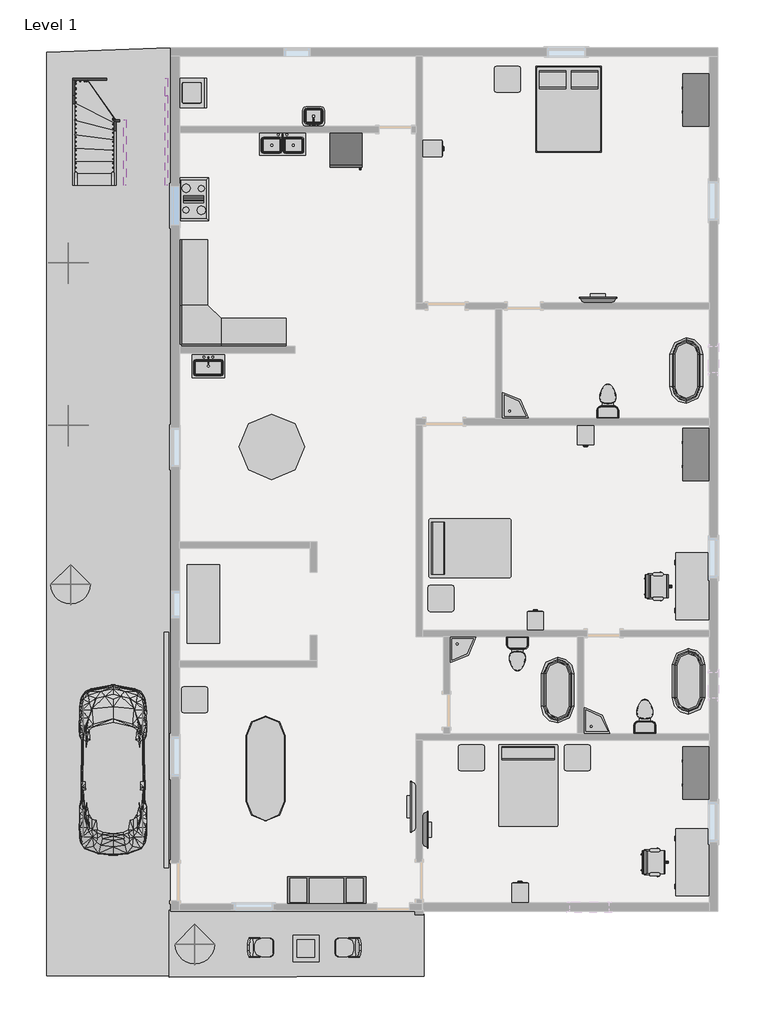
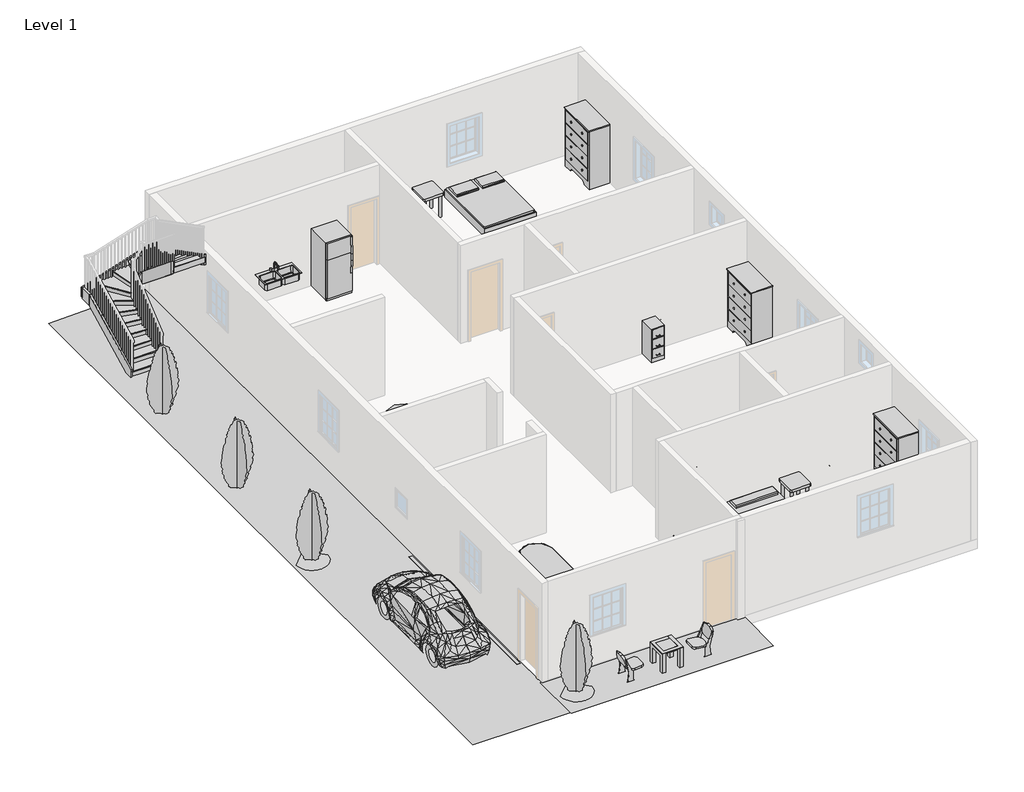
# One storey, part 3 of 3: 30 furniture elements, 16 flow terminals, 8 members, 7 proxies, 4 geographic elements, 1 stair flight.
"""IFC4 building model written with IfcOpenShell, lengths in millimetres."""

from ifc_helpers import new_model, si_unit, frame, origin, place, context, project, spatial, polyline, outline, extrude, triangles, transform, mapped, element, save
from components import proxy_bb1e6e30, parking_space_9_x_18_90_deg_b8b21359, rpc_beetle_rpc_beetle_3ce7ba48, proxy_a13a33b2, proxy_718fa39f, flow_terminal_accce45a, flow_terminal_bd5cdcf8, flow_terminal_a53be723, flow_terminal_38af2918, flow_terminal_62a433f7, toilet_domestic_3d_toilet_domestic_3d_f7549cf7, toilet_domestic_3d_toilet_domestic_3d_183bbd19, flow_terminal_b374fae2, furniture_1d2926bd, furniture_0253826f, furniture_552c1472, chair_task_arms_chair_task_arms_fa5a08ef, furniture_013ab306, furniture_9fa109b2, furniture_cf0b6580, furniture_3d1d9cbc, furniture_56245f3a, furniture_d9bcc661, furniture_b5c51a22, furniture_e05f6f82, furniture_bbcc68ce, furniture_bcf351fa, furniture_a5b052b6, furniture_45e3acac, rpc_tree_conifer_chinese_juniper_7_1b9786cd, stair_flight_3c83121e

model = new_model("IFC4")

# Units and contexts
model_context = context("Model", 3, world=origin())
ifc_project = project(units=[si_unit("LENGTHUNIT", "METRE", prefix="MILLI")], contexts=[model_context])

# Site, building, storey
site = spatial("IfcSite", under=ifc_project)
building = spatial("IfcBuilding", under=site)
storey = spatial("IfcBuildingStorey", under=building, Name="Level 1", Elevation=0.0)

# Proxies
placement = place(None, origin())
element("IfcBuildingElementProxy", 1, Name="Building Element Proxy", at=placement, inside=storey, context=model_context, shape_type="Tessellation", body=[
    triangles([(-11126.0162292, -5278.538269, 0.0), (-5181.8354507, -5380.1378815, 0.0), (-5181.8354507, -6815.2380753, 0.0), (-11126.0162292, -6841.2184662, 0.0), (-5207.2356445, -5303.9378815, 0.0), (-5448.5354507, -5278.538269, 0.0), (-11096.8610321, -5272.1880753, 0.0), (-9567.1218475, -5278.538269, 0.0)], [[4, 8, 7], [8, 4, 3], [7, 1, 4], [8, 6, 7], [3, 2, 6], [5, 6, 2], [3, 6, 8]], closed=False),
])
element("IfcBuildingElementProxy", 2, Name="Building Element Proxy", at=placement, inside=storey, context=model_context, shape_type="Tessellation", body=[
    triangles([(-11087.3360321, 14812.8621185, 0.0), (-13982.9360321, 14711.2625061, 0.0), (-11100.035257, -6815.2380753, 0.0), (-13982.9360321, -6802.538269, 0.0)], [[2, 4, 3], [3, 1, 2]], closed=False),
])
proxy_shape = proxy_bb1e6e30(model_context)
element("IfcBuildingElementProxy", 3, Name="Cook Top-4 Unit : 36\" x 20\"", ObjectType="Cook Top-4 Unit : 36\" x 20\"", at=placement, inside=storey, context=model_context, shape_type="MappedRepresentation", body=[
    mapped(proxy_shape, transform((-10553.9357228, 11282.2620171, 0.0), x_axis=(0.0, 1.0000000000000002, 0.0), y_axis=(-1.0000000000000002, 0.0, 0.0), z_axis=(0.0, 0.0, 1.0))),
])
parking_space_9_x_18_90_deg_shape = parking_space_9_x_18_90_deg_b8b21359(model_context)
element("IfcBuildingElementProxy", 4, Name="Parking Space : 9' x 18' - 90 deg", ObjectType="Parking Space : 9' x 18' - 90 deg", at=placement, inside=storey, context=model_context, shape_type="MappedRepresentation", body=[
    mapped(parking_space_9_x_18_90_deg_shape, transform((-11188.9357228, -4287.9379829, 0.0), x_axis=(-1.0, 0.0, 0.0), y_axis=(0.0, -1.0, 0.0), z_axis=(0.0, 0.0, 1.0))),
])
rpc_beetle_rpc_beetle_shape = rpc_beetle_rpc_beetle_3ce7ba48(model_context)
element("IfcBuildingElementProxy", 5, Name="RPC Beetle : RPC Beetle", ObjectType="RPC Beetle : RPC Beetle", at=placement, inside=storey, context=model_context, shape_type="MappedRepresentation", body=[
    mapped(rpc_beetle_rpc_beetle_shape, transform((-12433.5357228, -3246.5379829, 0.0), x_axis=(1.0000000000000007, 0.0, 0.0), y_axis=(0.0, 1.0000000000000007, 0.0), z_axis=(0.0, 0.0, 1.0))),
])
proxy_2_shape = proxy_a13a33b2(model_context)
element("IfcBuildingElementProxy", 6, Name="Refrigerator : 30\" x 32\" RH", ObjectType="Refrigerator : 30\" x 32\" RH", at=placement, inside=storey, context=model_context, shape_type="MappedRepresentation", body=[
    mapped(proxy_2_shape, transform((-7005.8732228, 12443.1130456, 0.0), x_axis=(1.0000000000000009, 0.0, 0.0), y_axis=(0.0, 1.0000000000000009, 0.0), z_axis=(0.0, 0.0, 1.0))),
])
proxy_3_shape = proxy_718fa39f(model_context)
element("IfcBuildingElementProxy", 7, Name="Washer : 27\" x 25\" x 35\"", ObjectType="Washer : 27\" x 25\" x 35\"", at=placement, inside=storey, context=model_context, shape_type="MappedRepresentation", body=[
    mapped(proxy_3_shape, transform((-10845.7852876, 14179.1794856, 0.0), x_axis=(0.0, -1.0000000000000004, 0.0), y_axis=(1.0000000000000004, 0.0, 0.0), z_axis=(0.0, 0.0, 1.0))),
])

# Flow terminals
flow_terminal_shape = flow_terminal_accce45a(model_context)
element("IfcFlowTerminal", 8, ObjectType="Floor Drain - Round : 5\" Strainer - 2\" Drain", at=placement, inside=storey, context=model_context, shape_type="MappedRepresentation", body=[
    mapped(flow_terminal_shape, transform((-10630.1357228, 14330.2620171, 0.0), x_axis=(1.0, 0.0, 0.0), y_axis=(0.0, 1.0, 0.0), z_axis=(0.0, 0.0, 1.0))),
])
element("IfcFlowTerminal", 9, ObjectType="Floor Drain - Round : 5\" Strainer - 2\" Drain", at=placement, inside=storey, context=model_context, shape_type="MappedRepresentation", body=[
    mapped(flow_terminal_shape, transform((230.9261263, 6530.9872371, 0.0), x_axis=(1.0, 0.0, 0.0), y_axis=(0.0, 1.0, 0.0), z_axis=(0.0, 0.0, 1.0))),
])
element("IfcFlowTerminal", 10, ObjectType="Floor Drain - Round : 5\" Strainer - 2\" Drain", at=placement, inside=storey, context=model_context, shape_type="MappedRepresentation", body=[
    mapped(flow_terminal_shape, transform((596.6642772, -833.5379829, 0.0), x_axis=(1.0, 0.0, 0.0), y_axis=(0.0, 1.0, 0.0), z_axis=(0.0, 0.0, 1.0))),
])
element("IfcFlowTerminal", 11, ObjectType="Floor Drain - Round : 5\" Strainer - 2\" Drain", at=placement, inside=storey, context=model_context, shape_type="MappedRepresentation", body=[
    mapped(flow_terminal_shape, transform((-2705.3357228, -909.7379829, 0.0), x_axis=(1.0, 0.0, 0.0), y_axis=(0.0, 1.0, 0.0), z_axis=(0.0, 0.0, 1.0))),
])
flow_terminal_2_shape = flow_terminal_bd5cdcf8(model_context)
element("IfcFlowTerminal", 12, ObjectType="Sink - Corner Floor : 24\"", at=placement, inside=storey, context=model_context, shape_type="MappedRepresentation", body=[
    mapped(flow_terminal_2_shape, transform((-3365.7357228, 6176.8620171, 609.6), x_axis=(1.0, 0.0, 0.0), y_axis=(0.0, 1.0, 0.0), z_axis=(0.0, 0.0, 1.0))),
])
element("IfcFlowTerminal", 13, ObjectType="Sink - Corner Floor : 24\"", at=placement, inside=storey, context=model_context, shape_type="MappedRepresentation", body=[
    mapped(flow_terminal_2_shape, transform((-4584.9357228, 1096.8620171, 609.6), x_axis=(0.0, -1.0000000000000004, 0.0), y_axis=(1.0000000000000004, 0.0, 0.0), z_axis=(0.0, 0.0, 1.0))),
])
element("IfcFlowTerminal", 14, ObjectType="Sink - Corner Floor : 24\"", at=placement, inside=storey, context=model_context, shape_type="MappedRepresentation", body=[
    mapped(flow_terminal_2_shape, transform((-1460.7357228, -1163.7379829, 609.6), x_axis=(1.0000000000000002, 0.0, 0.0), y_axis=(0.0, 1.0000000000000002, 0.0), z_axis=(0.0, 0.0, 1.0))),
])
flow_terminal_3_shape = flow_terminal_a53be723(model_context)
element("IfcFlowTerminal", 15, ObjectType="Sink Kitchen-Double : 42\" x 21\"", at=placement, inside=storey, context=model_context, shape_type="MappedRepresentation", body=[
    mapped(flow_terminal_3_shape, transform((-8499.5249633, 12575.316616, 0.0), x_axis=(1.0, 0.0, 0.0), y_axis=(0.0, 1.0, 0.0), z_axis=(0.0, 0.0, 1.0))),
])
flow_terminal_4_shape = flow_terminal_38af2918(model_context)
element("IfcFlowTerminal", 16, ObjectType="Sink Kitchen-Single : 30\" x 21\"", at=placement, inside=storey, context=model_context, shape_type="MappedRepresentation", body=[
    mapped(flow_terminal_4_shape, transform((-10226.7249633, 7393.716616, 0.0), x_axis=(1.0, 0.0, 0.0), y_axis=(0.0, 1.0, 0.0), z_axis=(0.0, 0.0, 1.0))),
])
flow_terminal_5_shape = flow_terminal_62a433f7(model_context)
element("IfcFlowTerminal", 17, ObjectType="Sink Vanity-Square : 20\" x 18\"", at=placement, inside=storey, context=model_context, shape_type="MappedRepresentation", body=[
    mapped(flow_terminal_5_shape, transform((-7744.2464822, 13164.2074182, 0.0), x_axis=(-1.0000000000000004, 0.0, 0.0), y_axis=(0.0, -1.0000000000000004, 0.0), z_axis=(0.0, 0.0, 1.0))),
])
toilet_domestic_3d_toilet_domestic_3d_shape = toilet_domestic_3d_toilet_domestic_3d_f7549cf7(model_context)
toilet_domestic_3d_toilet_domestic_3d_2_shape = toilet_domestic_3d_toilet_domestic_3d_183bbd19(model_context)
element("IfcFlowTerminal", 18, ObjectType="Toilet-Domestic-3D : Toilet-Domestic-3D", at=placement, inside=storey, context=model_context, shape_type="MappedRepresentation", body=[
    mapped(toilet_domestic_3d_toilet_domestic_3d_shape, transform((-901.9357228, 6671.5580445, 0.0), x_axis=(-0.9999999999999998, 0.0, 0.0), y_axis=(0.0, -0.9999999999999998, 0.0), z_axis=(0.0, 0.0, 1.0))),
    mapped(toilet_domestic_3d_toilet_domestic_3d_2_shape, transform((-901.9357228, 6671.5580445, 0.0), x_axis=(-0.9999999999999998, 0.0, 0.0), y_axis=(0.0, -0.9999999999999998, 0.0), z_axis=(0.0, 0.0, 1.0))),
])
element("IfcFlowTerminal", 19, ObjectType="Toilet-Domestic-3D : Toilet-Domestic-3D", at=placement, inside=storey, context=model_context, shape_type="MappedRepresentation", body=[
    mapped(toilet_domestic_3d_toilet_domestic_3d_shape, transform((-3010.1357228, 602.1659898, 0.0), x_axis=(1.0, 0.0, 0.0), y_axis=(0.0, 1.0, 0.0), z_axis=(0.0, 0.0, 1.0))),
    mapped(toilet_domestic_3d_toilet_domestic_3d_2_shape, transform((-3010.1357228, 602.1659898, 0.0), x_axis=(1.0, 0.0, 0.0), y_axis=(0.0, 1.0, 0.0), z_axis=(0.0, 0.0, 1.0))),
])
element("IfcFlowTerminal", 20, ObjectType="Toilet-Domestic-3D : Toilet-Domestic-3D", at=placement, inside=storey, context=model_context, shape_type="MappedRepresentation", body=[
    mapped(toilet_domestic_3d_toilet_domestic_3d_shape, transform((-38.3357228, -669.0419555, 0.0), x_axis=(-1.0000000000000004, 0.0, 0.0), y_axis=(0.0, -1.0000000000000004, 0.0), z_axis=(0.0, 0.0, 1.0))),
    mapped(toilet_domestic_3d_toilet_domestic_3d_2_shape, transform((-38.3357228, -669.0419555, 0.0), x_axis=(-1.0000000000000004, 0.0, 0.0), y_axis=(0.0, -1.0000000000000004, 0.0), z_axis=(0.0, 0.0, 1.0))),
])
flow_terminal_6_shape = flow_terminal_b374fae2(model_context)
element("IfcFlowTerminal", 21, ObjectType="Tub-Free Standing-3D : 30\" x 60\"", at=placement, inside=storey, context=model_context, shape_type="MappedRepresentation", body=[
    mapped(flow_terminal_6_shape, transform((926.8642772, 7294.4620171, 0.0), x_axis=(1.0, 0.0, 0.0), y_axis=(0.0, 1.0, 0.0), z_axis=(0.0, 0.0, 1.0))),
])
element("IfcFlowTerminal", 22, ObjectType="Tub-Free Standing-3D : 30\" x 60\"", at=placement, inside=storey, context=model_context, shape_type="MappedRepresentation", body=[
    mapped(flow_terminal_6_shape, transform((-2070.3357228, -147.7379829, 0.0), x_axis=(1.0, 0.0, 0.0), y_axis=(0.0, 1.0, 0.0), z_axis=(0.0, 0.0, 1.0))),
])
element("IfcFlowTerminal", 23, ObjectType="Tub-Free Standing-3D : 30\" x 60\"", at=placement, inside=storey, context=model_context, shape_type="MappedRepresentation", body=[
    mapped(flow_terminal_6_shape, transform((977.6642772, 55.4620171, 0.0), x_axis=(1.0, 0.0, 0.0), y_axis=(0.0, 1.0, 0.0), z_axis=(0.0, 0.0, 1.0))),
])

# Furniture
furniture_shape = furniture_1d2926bd(model_context)
element("IfcFurniture", 24, ObjectType="Bed-Box : Queen 60\" x 79\"", at=placement, inside=storey, context=model_context, shape_type="MappedRepresentation", body=[
    mapped(furniture_shape, transform((-2155.4881818, 13612.1915253, 0.0), x_axis=(1.0, 0.0, 0.0), y_axis=(0.0, 1.0, 0.0), z_axis=(0.0, 0.0, 1.0))),
])
furniture_2_shape = furniture_0253826f(model_context)
element("IfcFurniture", 25, ObjectType="Bed-Standard.0001 : Double 54\" x 75\"", at=placement, inside=storey, context=model_context, shape_type="MappedRepresentation", body=[
    mapped(furniture_2_shape, transform((-4160.6308048, 2882.7734925, 0.0), x_axis=(0.0, 1.0000000000000002, 0.0), y_axis=(-1.0000000000000002, 0.0, 0.0), z_axis=(0.0, 0.0, 1.0))),
])
element("IfcFurniture", 26, ObjectType="Bed-Standard.0001 : Double 54\" x 75\"", at=placement, inside=storey, context=model_context, shape_type="MappedRepresentation", body=[
    mapped(furniture_2_shape, transform((-3027.6242474, -2324.6429009, 0.0), x_axis=(1.0, 0.0, 0.0), y_axis=(0.0, 1.0, 0.0), z_axis=(0.0, 0.0, 1.0))),
])
furniture_3_shape = furniture_552c1472(model_context)
element("IfcFurniture", 27, ObjectType="Cabinet-File 3 Drawer : 15\" x 18\"", at=placement, inside=storey, context=model_context, shape_type="MappedRepresentation", body=[
    mapped(furniture_3_shape, transform((-5133.4700229, 12591.2584641, 0.0), x_axis=(0.0, 1.0000000000000002, 0.0), y_axis=(-1.0000000000000002, 0.0, 0.0), z_axis=(0.0, 0.0, 1.0))),
])
element("IfcFurniture", 28, ObjectType="Cabinet-File 3 Drawer : 15\" x 18\"", at=placement, inside=storey, context=model_context, shape_type="MappedRepresentation", body=[
    mapped(furniture_3_shape, transform((-2718.9321698, 1310.327717, 0.0), x_axis=(-1.0000000000000002, 0.0, 0.0), y_axis=(0.0, -1.0000000000000002, 0.0), z_axis=(0.0, 0.0, 1.0))),
])
element("IfcFurniture", 29, ObjectType="Cabinet-File 3 Drawer : 15\" x 18\"", at=placement, inside=storey, context=model_context, shape_type="MappedRepresentation", body=[
    mapped(furniture_3_shape, transform((-1294.7392757, 5937.9963172, 0.0), x_axis=(1.0, 0.0, 0.0), y_axis=(0.0, 1.0, 0.0), z_axis=(0.0, 0.0, 1.0))),
])
element("IfcFurniture", 30, ObjectType="Cabinet-File 3 Drawer : 15\" x 18\"", at=placement, inside=storey, context=model_context, shape_type="MappedRepresentation", body=[
    mapped(furniture_3_shape, transform((-3074.5321698, -5014.272283, 0.0), x_axis=(-1.0, 0.0, 0.0), y_axis=(0.0, -1.0, 0.0), z_axis=(0.0, 0.0, 1.0))),
])
chair_task_arms_chair_task_arms_shape = chair_task_arms_chair_task_arms_fa5a08ef(model_context)
element("IfcFurniture", 31, ObjectType="Chair-Task Arms : Chair-Task Arms", at=placement, inside=storey, context=model_context, shape_type="MappedRepresentation", body=[
    mapped(chair_task_arms_chair_task_arms_shape, transform((222.1183756, 2406.2528368, 0.0), x_axis=(0.0, -1.0000000000000004, 0.0), y_axis=(1.0000000000000004, 0.0, 0.0), z_axis=(0.0, 0.0, 1.0))),
])
element("IfcFurniture", 32, ObjectType="Chair-Task Arms : Chair-Task Arms", at=placement, inside=storey, context=model_context, shape_type="MappedRepresentation", body=[
    mapped(chair_task_arms_chair_task_arms_shape, transform((145.9183756, -4019.9471632, 0.0), x_axis=(0.0, -1.0000000000000004, 0.0), y_axis=(1.0000000000000004, 0.0, 0.0), z_axis=(0.0, 0.0, 1.0))),
])
furniture_4_shape = furniture_013ab306(model_context)
element("IfcFurniture", 33, ObjectType="Desk : 60\" x 30\"", at=placement, inside=storey, context=model_context, shape_type="MappedRepresentation", body=[
    mapped(furniture_4_shape, transform((698.2642772, 3027.2620171, 0.0), x_axis=(0.0, -1.0000000000000007, 0.0), y_axis=(1.0000000000000007, 0.0, 0.0), z_axis=(0.0, 0.0, 1.0))),
])
element("IfcFurniture", 34, ObjectType="Desk : 60\" x 30\"", at=placement, inside=storey, context=model_context, shape_type="MappedRepresentation", body=[
    mapped(furniture_4_shape, transform((698.2642772, -3398.9379829, 0.0), x_axis=(0.0, -1.0000000000000004, 0.0), y_axis=(1.0000000000000004, 0.0, 0.0), z_axis=(0.0, 0.0, 1.0))),
])
furniture_5_shape = furniture_9fa109b2(model_context)
element("IfcFurniture", 35, ObjectType="Dresser : 48\" x 72\" x 24\"", at=placement, inside=storey, context=model_context, shape_type="MappedRepresentation", body=[
    mapped(furniture_5_shape, transform((1518.6272313, 13324.4687573, 0.0), x_axis=(0.0, -1.0000000000000007, 0.0), y_axis=(1.0000000000000007, 0.0, 0.0), z_axis=(0.0, 0.0, 1.0))),
])
element("IfcFurniture", 36, ObjectType="Dresser : 48\" x 72\" x 24\"", at=placement, inside=storey, context=model_context, shape_type="MappedRepresentation", body=[
    mapped(furniture_5_shape, transform((1518.6272313, 5069.4687573, 0.0), x_axis=(0.0, -1.0000000000000007, 0.0), y_axis=(1.0000000000000007, 0.0, 0.0), z_axis=(0.0, 0.0, 1.0))),
])
element("IfcFurniture", 37, ObjectType="Dresser : 48\" x 72\" x 24\"", at=placement, inside=storey, context=model_context, shape_type="MappedRepresentation", body=[
    mapped(furniture_5_shape, transform((1518.6272313, -2347.3312427, 0.0), x_axis=(0.0, -1.0000000000000007, 0.0), y_axis=(1.0000000000000007, 0.0, 0.0), z_axis=(0.0, 0.0, 1.0))),
])
furniture_6_shape = furniture_cf0b6580(model_context)
element("IfcFurniture", 38, ObjectType="Entertainment Center : 72\" x 72\" x 24\"", at=placement, inside=storey, context=model_context, shape_type="MappedRepresentation", body=[
    mapped(furniture_6_shape, transform((-7455.1357228, -4389.5379829, 0.0), x_axis=(1.0, 0.0, 0.0), y_axis=(0.0, 1.0, 0.0), z_axis=(0.0, 0.0, 1.0))),
])
furniture_7_shape = furniture_3d1d9cbc(model_context)
element("IfcFurniture", 39, ObjectType="Seating-Auditorium : 18\" x 24\" x 30\"", at=placement, inside=storey, context=model_context, shape_type="MappedRepresentation", body=[
    mapped(furniture_7_shape, transform((-9194.4111326, -5981.410114, 0.0), x_axis=(0.0, -1.0000000000000007, 0.0), y_axis=(1.0000000000000007, 0.0, 0.0), z_axis=(0.0, 0.0, 1.0))),
])
element("IfcFurniture", 40, ObjectType="Seating-Auditorium : 18\" x 24\" x 30\"", at=placement, inside=storey, context=model_context, shape_type="MappedRepresentation", body=[
    mapped(furniture_7_shape, transform((-6757.2603129, -6302.8658517, 0.0), x_axis=(0.0, 1.000000000000001, 0.0), y_axis=(-1.000000000000001, 0.0, 0.0), z_axis=(0.0, 0.0, 1.0))),
])
furniture_8_shape = furniture_56245f3a(model_context)
element("IfcFurniture", 41, ObjectType="TV - Flat Screen : 32\"", at=placement, inside=storey, context=model_context, shape_type="MappedRepresentation", body=[
    mapped(furniture_8_shape, transform((-5161.3970991, -3394.9934687, 914.4), x_axis=(0.0, 1.0, 0.0), y_axis=(-1.0, 0.0, 0.0), z_axis=(0.0, 0.0, 1.0))),
])
element("IfcFurniture", 42, ObjectType="TV - Flat Screen : 32\"", at=placement, inside=storey, context=model_context, shape_type="MappedRepresentation", body=[
    mapped(furniture_8_shape, transform((-1134.4802369, 8927.8006408, 914.4), x_axis=(-1.0, 0.0, 0.0), y_axis=(0.0, -1.0, 0.0), z_axis=(0.0, 0.0, 1.0))),
])
furniture_9_shape = furniture_d9bcc661(model_context)
element("IfcFurniture", 43, ObjectType="TV - Flat Screen : 46\"", at=placement, inside=storey, context=model_context, shape_type="MappedRepresentation", body=[
    mapped(furniture_9_shape, transform((-5430.8743464, -2869.482497, 0.0), x_axis=(0.0, -1.0000000000000004, 0.0), y_axis=(1.0000000000000004, 0.0, 0.0), z_axis=(0.0, 0.0, 1.0))),
])
furniture_10_shape = furniture_b5c51a22(model_context)
element("IfcFurniture", 44, ObjectType="Table-Coffee : 24\" x 24\" x 24\"", at=placement, inside=storey, context=model_context, shape_type="MappedRepresentation", body=[
    mapped(furniture_10_shape, transform((-7956.0014895, -6262.7490607, 0.0), x_axis=(1.0, 0.0, 0.0), y_axis=(0.0, 1.0, 0.0), z_axis=(0.0, 0.0, 1.0))),
])
furniture_11_shape = furniture_e05f6f82(model_context)
element("IfcFurniture", 45, ObjectType="Table-Dining Oval : 36\" x 96\" Glass Top", at=placement, inside=storey, context=model_context, shape_type="MappedRepresentation", body=[
    mapped(furniture_11_shape, transform((-9235.6340834, -1574.7183108, 0.0), x_axis=(0.0, 1.0000000000000002, 0.0), y_axis=(-1.0000000000000002, 0.0, 0.0), z_axis=(0.0, 0.0, 1.0))),
])
furniture_12_shape = furniture_bbcc68ce(model_context)
element("IfcFurniture", 46, ObjectType="Table-Dining Round w Chairs : 60\" Diameter", at=placement, inside=storey, context=model_context, shape_type="MappedRepresentation", body=[
    mapped(furniture_12_shape, transform((-8837.1230967, 5701.3407056, 0.0), x_axis=(1.0, 0.0, 0.0), y_axis=(0.0, 1.0, 0.0), z_axis=(0.0, 0.0, 1.0))),
])
furniture_13_shape = furniture_bcf351fa(model_context)
element("IfcFurniture", 47, ObjectType="Table-End : 24\" x 24\"", at=placement, inside=storey, context=model_context, shape_type="MappedRepresentation", body=[
    mapped(furniture_13_shape, transform((-3547.2693531, 13923.8620171, 0.0), x_axis=(1.0, 0.0, 0.0), y_axis=(0.0, 1.0, 0.0), z_axis=(0.0, 0.0, 1.0))),
])
element("IfcFurniture", 48, ObjectType="Table-End : 24\" x 24\"", at=placement, inside=storey, context=model_context, shape_type="MappedRepresentation", body=[
    mapped(furniture_13_shape, transform((-5096.6693531, 1833.4620171, 0.0), x_axis=(1.0, 0.0, 0.0), y_axis=(0.0, 1.0, 0.0), z_axis=(0.0, 0.0, 1.0))),
])
element("IfcFurniture", 49, ObjectType="Table-End : 24\" x 24\"", at=placement, inside=storey, context=model_context, shape_type="MappedRepresentation", body=[
    mapped(furniture_13_shape, transform((-4385.4693531, -1874.9379829, 0.0), x_axis=(1.0, 0.0, 0.0), y_axis=(0.0, 1.0, 0.0), z_axis=(0.0, 0.0, 1.0))),
])
element("IfcFurniture", 50, ObjectType="Table-End : 24\" x 24\"", at=placement, inside=storey, context=model_context, shape_type="MappedRepresentation", body=[
    mapped(furniture_13_shape, transform((-1921.6693531, -1874.9379829, 0.0), x_axis=(1.0, 0.0, 0.0), y_axis=(0.0, 1.0, 0.0), z_axis=(0.0, 0.0, 1.0))),
])
element("IfcFurniture", 51, ObjectType="Table-End : 24\" x 24\"", at=placement, inside=storey, context=model_context, shape_type="MappedRepresentation", body=[
    mapped(furniture_13_shape, transform((-10837.0693531, -528.7379829, 0.0), x_axis=(1.0, 0.0, 0.0), y_axis=(0.0, 1.0, 0.0), z_axis=(0.0, 0.0, 1.0))),
])
furniture_14_shape = furniture_a5b052b6(model_context)
element("IfcFurniture", 52, ObjectType="Table-Rectangular : 72\" x 30\"", at=placement, inside=storey, context=model_context, shape_type="MappedRepresentation", body=[
    mapped(furniture_14_shape, transform((-10325.3357228, 1858.8620171, 0.0), x_axis=(0.0, 1.0000000000000002, 0.0), y_axis=(-1.0000000000000002, 0.0, 0.0), z_axis=(0.0, 0.0, 1.0))),
])
furniture_15_shape = furniture_45e3acac(model_context)
element("IfcFurniture", 53, ObjectType="Work Station Cubicle : 96\" x 96\"", at=placement, inside=storey, context=model_context, shape_type="MappedRepresentation", body=[
    mapped(furniture_15_shape, transform((-11379.1587304, 7984.9937693, 0.0), x_axis=(0.0, 1.0000000000000002, 0.0), y_axis=(-1.0000000000000002, 0.0, 0.0), z_axis=(0.0, 0.0, 1.0))),
])

# Geographic elements
rpc_tree_conifer_chinese_juniper_7_shape = rpc_tree_conifer_chinese_juniper_7_1b9786cd(model_context)
element("IfcGeographicElement", 54, ObjectType="RPC Tree - Conifer : Chinese Juniper - 7'", at=placement, inside=storey, context=model_context, shape_type="MappedRepresentation", body=[
    mapped(rpc_tree_conifer_chinese_juniper_7_shape, transform((-10528.7323939, -6065.9379829, 0.0), x_axis=(1.0, 0.0, 0.0), y_axis=(0.0, 1.0, 0.0), z_axis=(0.0, 0.0, 1.0))),
])
element("IfcGeographicElement", 55, ObjectType="RPC Tree - Conifer : Chinese Juniper - 7'", at=placement, inside=storey, context=model_context, shape_type="MappedRepresentation", body=[
    mapped(rpc_tree_conifer_chinese_juniper_7_shape, transform((-13475.1323939, 9809.0620171, 0.0), x_axis=(1.0, 0.0, 0.0), y_axis=(0.0, 1.0, 0.0), z_axis=(0.0, 0.0, 1.0))),
])
element("IfcGeographicElement", 56, ObjectType="RPC Tree - Conifer : Chinese Juniper - 7'", at=placement, inside=storey, context=model_context, shape_type="MappedRepresentation", body=[
    mapped(rpc_tree_conifer_chinese_juniper_7_shape, transform((-13475.1323939, 6024.4620171, 0.0), x_axis=(1.0, 0.0, 0.0), y_axis=(0.0, 1.0, 0.0), z_axis=(0.0, 0.0, 1.0))),
])
element("IfcGeographicElement", 57, ObjectType="RPC Tree - Conifer : Chinese Juniper - 7'", at=placement, inside=storey, context=model_context, shape_type="MappedRepresentation", body=[
    mapped(rpc_tree_conifer_chinese_juniper_7_shape, transform((-13424.3323939, 2316.0620171, 0.0), x_axis=(1.0, 0.0, 0.0), y_axis=(0.0, 1.0, 0.0), z_axis=(0.0, 0.0, 1.0))),
])

# Members
element("IfcMember", 58, ObjectType="Stringer - 2\" Width", at=placement, inside=storey, context=model_context, shape_type="SweptSolid", body=[
    extrude(outline(polyline([(11608.7303252, 0.0), (11608.7303252, 229.639954), (13696.1475169, 1305.3956453), (13696.1475169, 962.500629), (11828.4926428, 0.0), (11608.7303252, 0.0)])), frame((-13373.3357228, 0.0, 0.0), z_axis=(1.0, 0.0, 0.0), x_axis=(0.0, 1.0, 0.0)), (0.0, 0.0, 1.0), 50.8),
])
element("IfcMember", 59, ObjectType="Stringer - 2\" Width", at=placement, inside=storey, context=model_context, shape_type="SweptSolid", body=[
    extrude(outline(polyline([(-13322.5357228, 13696.1475169), (-13373.3357228, 13696.1475169), (-13373.3357228, 14050.8620171), (-13322.5357228, 14050.8620171), (-13322.5357228, 13696.1475169)])), frame((0.0, 0.0, 962.500629), z_axis=(0.0, 0.0, 1.0), x_axis=(1.0, 0.0, 0.0)), (0.0, 0.0, 1.0), 342.8950162),
])
element("IfcMember", 60, ObjectType="Stringer - 2\" Width", at=placement, inside=storey, context=model_context, shape_type="SweptSolid", body=[
    extrude(outline(polyline([(1289.0952212, -13373.3357228), (1000.5956453, -13373.3357228), (1000.5956453, -13203.8132398), (1638.9682298, -11214.3357228), (1969.9972697, -11214.3357228), (1969.9972697, -11251.3158401), (1289.0952212, -13373.3357228)])), frame((0.0, 14050.8620171, 0.0), z_axis=(0.0, 1.0, 0.0), x_axis=(0.0, 0.0, 1.0)), (0.0, 0.0, 1.0), 50.8),
])
element("IfcMember", 61, ObjectType="Stringer - 2\" Width", at=placement, inside=storey, context=model_context, shape_type="SweptSolid", body=[
    extrude(outline(polyline([(-11214.3357228, 14101.6620171), (-11163.5357228, 14101.6620171), (-11163.5357228, 13696.1475169), (-11214.3357228, 13696.1475169), (-11214.3357228, 14101.6620171)])), frame((0.0, 0.0, 1649.8904473), z_axis=(0.0, 0.0, 1.0), x_axis=(1.0, 0.0, 0.0)), (0.0, 0.0, 1.0), 320.1068224),
])
element("IfcMember", 62, ObjectType="Stringer - 2\" Width", at=placement, inside=storey, context=model_context, shape_type="SweptSolid", body=[
    extrude(outline(polyline([(13696.1475169, 1969.9972697), (13696.1475169, 1649.8904473), (11608.7303252, 2725.6461385), (11608.7303252, 3045.7529609), (13696.1475169, 1969.9972697)])), frame((-11214.3357228, 0.0, 0.0), z_axis=(1.0, 0.0, 0.0), x_axis=(0.0, 1.0, 0.0)), (0.0, 0.0, 1.0), 50.8),
])
element("IfcMember", 63, ObjectType="Stringer - 2\" Width", at=placement, inside=storey, context=model_context, shape_type="SweptSolid", body=[
    extrude(outline(polyline([(11608.7303252, 0.0), (11608.7303252, 176.1764461), (13085.6620171, 1380.418648), (13085.6620171, 987.1410923), (11874.9919698, 0.0), (11608.7303252, 0.0)])), frame((-12408.1357228, 0.0, 0.0), z_axis=(1.0, 0.0, 0.0), x_axis=(0.0, 1.0, 0.0)), (0.0, 0.0, 1.0), 50.8),
])
element("IfcMember", 64, ObjectType="Stringer - 2\" Width", at=placement, inside=storey, context=model_context, shape_type="SweptSolid", body=[
    extrude(outline(polyline([(1573.2682978, -12408.1357228), (1028.5617647, -12408.1357228), (1028.5617647, -12373.8935055), (1360.465107, -12179.5357228), (1926.1409689, -12179.5357228), (1926.1409689, -12201.4986054), (1573.2682978, -12408.1357228)])), frame((0.0, 13085.6620171, 0.0), z_axis=(0.0, 1.0, 0.0), x_axis=(0.0, 0.0, 1.0)), (0.0, 0.0, 1.0), 50.8),
])
element("IfcMember", 65, ObjectType="Stringer - 2\" Width", at=placement, inside=storey, context=model_context, shape_type="SweptSolid", body=[
    extrude(outline(polyline([(13136.4620171, 1926.1409689), (13136.4620171, 1532.8634131), (11608.7303252, 2778.5262875), (11608.7303252, 3171.8038432), (13136.4620171, 1926.1409689)])), frame((-12179.5357228, 0.0, 0.0), z_axis=(1.0, 0.0, 0.0), x_axis=(0.0, 1.0, 0.0)), (0.0, 0.0, 1.0), 50.8),
])

# Stair flight
stair_flight_shape = stair_flight_3c83121e(model_context)
element("IfcStairFlight", 66, ObjectType="2\" Tread 1\" Nosing 1/4\" Riser", at=placement, inside=storey, context=model_context, shape_type="MappedRepresentation", body=[
    mapped(stair_flight_shape, transform((0.0, 0.0, 0.0), x_axis=(1.0, 0.0, 0.0), y_axis=(0.0, 1.0, 0.0), z_axis=(0.0, 0.0, 1.0))),
])

save(model, "model.ifc")

# Revit data of these elements
# Type "Cook Top-4 Unit : 36\" x 20\""
#   Assembly Code = "E1090400"
#   Depth = 2' - 0"
#   Width = 3' - 0"
#   Burner Material = Steel, Chrome Plated
#   Cooktop Material = Steel, Polished
#   Default Elevation = 0
# Type "Parking Space : 9' x 18' - 90 deg"
#   Angle = 90.00°
#   Parking Length = 18' - 0"
#   Parking Width = 9' - 0"
#   pl = 18' - 0"
#   pw = 9' - 0"
# Type "RPC Beetle : RPC Beetle"
#   built-in parameter 1005195 = "RPC-16-0U6E-L4EG-ENH1-J3KF-SVEL-0TX4-C0"
#   Height = 0
# Type "Refrigerator : 30\" x 32\" RH"
#   Label = "REF."
#   Assembly Code = "E1090400"
#   Depth = 2' - 7 3/4"
#   Handle = 2' - 3"
#   Height = 5' - 10"
#   Rear Clearance = 0' - 2"
#   Top Door Height = 1' - 8"
#   Width = 2' - 5 3/8"
#   Material = Steel, Paint Finish, Ivory, Glossy
#   Default Elevation = 0
# Type "Washer : 27\" x 25\" x 35\""
#   Label = "W"
#   Assembly Code = "E1090400"
#   Depth = 2' - 1"
#   Height = 2' - 11"
#   Width = 2' - 3"
#   Washer Material = Steel, Paint Finish, Ivory, Matte
#   Default Elevation = 0
# Type "Floor Drain - Round : 5\" Strainer - 2\" Drain"
#   WFU = 2
#   Strainer Height = 0' - 3 1/4"
#   Strainer Radius = 0' - 2 1/2"
#   Strainer Diameter = 0' - 5"
#   Radius 6 = 0' - 0 5/8"
#   Radius 5 = 0' - 1 1/4"
#   Radius 4 = 0' - 1 7/8"
#   Radius 2 = 0' - 3.04167"
#   Radius 1 = 0' - 2.02083"
#   Radius 3 = 0' - 2 1/32"
#   Pipe Radius = 1"
#   Pipe Diameter = 2"
#   Height 2 = 0' - 0.725"
#   Height 1 = 0' - 1 13/16"
#   Body Radius = 0' - 4 1/16"
#   Body Height = 0' - 3 5/8"
#   Body Diameter = 0' - 8 1/8"
#   Drain Material = none
#   HWFU = 0
#   Default Elevation = 0
#   CWFU = 0
# Type "Sink - Corner Floor : 24\""
#   WFU = 2
#   Sink Radius = 2' - 0"
#   Sink Depth = 0' - 3 1/2"
#   Sanitary Radius = 3/4"
#   Sanitary Diameter = 1 1/2"
#   Radius 1 = 1' - 10"
#   Edge Width = 0' - 2"
#   Sink Material = none
#   HWFU = 0
#   Default Elevation = 0
#   CWFU = 0
# Type "Sink Kitchen-Double : 42\" x 21\""
#   Assembly Code = "D2010410"
#   Counter Height = 3' - 0"
#   Depth = 1' - 9"
#   Width = 3' - 6"
#   Faucet Material = Steel, Polished
#   Sink Material = Steel, Polished
#   Default Elevation = 0
# Type "Sink Kitchen-Single : 30\" x 21\""
#   Assembly Code = "D2010410"
#   Counter Height = 3' - 0"
#   Depth = 1' - 9"
#   Width = 2' - 6"
#   Faucet Material = Steel, Polished
#   Sink Material = Steel, Polished
#   Default Elevation = 0
# Type "Sink Vanity-Square : 20\" x 18\""
#   Assembly Code = "D2010400"
#   Counter Height = 2' - 7"
#   Depth = 1' - 6"
#   Width = 1' - 8"
#   Basin Material = Porcelain, Linen
#   Faucet Material = Steel, Polished
#   Default Elevation = 0
# Type "Toilet-Domestic-3D : Toilet-Domestic-3D"
#   Assembly Code = "D2010110"
#   Toilet - Bowl/Basin Material = Porcelain, Linen
#   Toilet - Seat Material = Laminate, Linen, Matte
#   Default Elevation = 0
# Type "Tub-Free Standing-3D : 30\" x 60\""
#   Assembly Code = "D2010110"
#   Height = 1' - 6"
#   Length = 5' - 0"
#   Width = 2' - 6"
#   Tub Material = Porcelain, Ivory
#   Default Elevation = 0
# Type "Bed-Box : Queen 60\" x 79\""
#   Assembly Code = "E2020200"
#   Length = 6' - 7"
#   Width = 5' - 0"
#   Frame Material = Birch
#   Mattress Material = Linen, White
#   Default Elevation = 0
# Type "Bed-Standard.0001 : Double 54\" x 75\""
#   Assembly Code = "E2020200"
#   Length = 6' - 3"
#   Width = 4' - 6"
#   Leg Material = Steel, Chrome Plated
#   Mattress Material = Linen, White
#   Default Elevation = 0
# Type "Cabinet-File 3 Drawer : 15\" x 18\""
#   Assembly Code = "E2020200"
#   Depth = 1' - 6"
#   Height = 3' - 5"
#   Width = 1' - 3"
#   Cabinet Material = Steel, Paint Finish, Ivory, Glossy
#   Handle Material = Steel, Chrome Plated
#   Default Elevation = 0
# Type "Chair-Task Arms : Chair-Task Arms"
#   Assembly Code = "E2020200"
#   Base Material = Plastic, Opaque Black
#   Caster Material = Plastic, Opaque Black
#   Seat/Back Material = Textile - Slate Blue
#   Default Elevation = 0
# Type "Desk : 60\" x 30\""
#   Assembly Code = "E2020200"
#   Depth = 2' - 6"
#   Height = 2' - 6"
#   Leg Height = 0' - 6"
#   Width = 5' - 0"
#   Body Material = Laminate, Ivory, Matte
#   Handle/Leg Material = Steel, Chrome Plated
#   Top Material = Cherry
#   Default Elevation = 0
# Type "Dresser : 48\" x 72\" x 24\""
#   Assembly Code = "E2020200"
#   Depth = 2' - 0"
#   Height = 6' - 0"
#   Width = 4' - 0"
#   Dresser Material = Laminate - Ivory, Glossy
#   Drawer Material = Laminate, Ivory, Matte
#   Knob Material = Cherry
#   Default Elevation = 0
# Type "Entertainment Center : 72\" x 72\" x 24\""
#   Assembly Code = "E2020200"
#   Center Width = 2' - 8"
#   Depth = 2' - 0"
#   Height = 6' - 0"
#   Width = 6' - 0"
#   Material = none
#   Default Elevation = 0
# Type "Seating-Auditorium : 18\" x 24\" x 30\""
#   Assembly Code = "E2020200"
#   Seat Material = Linen, Beige
#   Frame Material = Steel, Paint Finish, Dark Gray, Matte
#   Default Elevation = 0
# Type "TV - Flat Screen : 32\""
#   SinAng = 0' - 0.0193"
#   L = 2' - 3.79372"
#   H = 1' - 3.6354"
#   Thickness = 0' - 4.33071"
#   Diagonal = 2' - 7.88976"
#   CosAng = 0' - 0.03431"
#   Stand [instance default] = yes
#   Default Elevation = 0
# Type "TV - Flat Screen : 46\""
#   SinAng = 0' - 0.0193"
#   L = 3' - 4.83276"
#   H = 1' - 10.97053"
#   Thickness = 0' - 4.33071"
#   Diagonal = 3' - 10.85039"
#   CosAng = 0' - 0.03431"
#   Stand [instance default] = yes
#   Default Elevation = 0
# Type "Table-Coffee : 24\" x 24\" x 24\""
#   Assembly Code = "E2020200"
#   Height = 2' - 0"
#   Length = 2' - 0"
#   Width = 2' - 0"
#   Top Material = none
#   Frame Material = none
#   Default Elevation = 0
# Type "Table-Dining Oval : 36\" x 96\" Glass Top"
#   Assembly Code = "E2020200"
#   Length = 8' - 0"
#   Width = 3' - 0"
#   Base Material = Steel, Chrome Plated
#   Top Material = Glass - Clear, Grey
#   Default Elevation = 0
#   Description = (empty or 0)
# Type "Table-Dining Round w Chairs : 60\" Diameter"
#   Assembly Code = "E2020200"
#   Radius = 2' - 6"
#   Diameter = 5' - 0"
#   Height = 2' - 6"
#   Chairs = 6
#   Base Material = Pine
#   Top Material = Laminate, Linen, Matte
#   Default Elevation = 0
# Type "Table-End : 24\" x 24\""
#   Assembly Code = "E2020200"
#   Height = 2' - 6"
#   Length = 2' - 0"
#   Width = 2' - 0"
#   Base Material = Birch
#   Top Material = Laminate, Ivory, Matte
#   Default Elevation = 0
# Type "Table-Rectangular : 72\" x 30\""
#   Assembly Code = "E2020200"
#   Height = 2' - 6"
#   Length = 6' - 0"
#   Width = 2' - 6"
#   Base Material = Birch
#   Top Material = Birch
#   Default Elevation = 0
# Type "Work Station Cubicle : 96\" x 96\""
#   Assembly Code = "E2020"
#   Desktop Height = 2' - 6"
#   Desktop1 Width = 2' - 0"
#   Desktop2 Width = 2' - 0"
#   Panel Height = 5' - 6"
#   Panel1 Length = 5' - 0"
#   Panel2 Length = 5' - 0"
#   Cube Panel Material = Textile - Light Gray
#   Work Top Material = Laminate, Ivory, Matte
#   Default Elevation = 0
# Type "RPC Tree - Conifer : Chinese Juniper - 7'"
#   built-in parameter 1005198 = "{2, 15},{39, RPC-16-FUM3-UUQ0-UBF0-N000-ST1L-LVER-AU},{1, 0},{1, 0},{2, 13},{1, 8},{5, Color},{1, 0},{1, 0},{3, 0.8},{3, 0.8},{3, 0.8},{1, 8},{7, BBoxMin},{1, 0},{1, 0},{1, 0},{1, 0},{1, 0},{1, 8},{7, BBoxMax},{1, 0},{1, 0},{1, 0},{1, 0},{1, 0},{2, 11},{9, RPCTypeId},{1, 0},{1, 0},{39, RPC-16-FUM3-UUQ0-UBF0-N000-ST1L-LVER-AU},{1, 6},{14, RPCPlantHeight},{1, 0},{1, 0},{1, 7},{2, 11},{7, keyword},{1, 0},{1, 0},{34, :RPCs:Trees [General]:Geometry:RPC},{2, 11},{8, category},{1, 0},{1, 0},{15, Trees [General]},{2, 11},{12, LocalizedUID},{1, 0},{1, 0},{15, Chinese Juniper},{2, 14},{6, Height},{1, 0},{1, 0},{1, 7},{1, 2},{16, Cast Reflections},{1, 0},{1, 0},{1, 0},{1, 2},{12, Cast Shadows},{1, 0},{1, 0},{1, 1},{1, 2},{9, Lock View},{1, 0},{1, 0},{1, 0},{1, 4},{5, ViewC},{1, 0},{1, 0},{1, 0},{21, assetlibrary_base.fbx},{1, 5},"
#   built-in parameter 1005195 = "RPC-16-FUM3-UUQ0-UBF0-N000-ST1L-LVER-AU"
#   Type Comments = "Chinese Juniper"
#   Assembly Code = "G2050500"
#   Height = 7' - 0"
#   Description = (empty or 0)
#   Default Elevation = 0
# Elements 1, 2 (IfcBuildingElementProxy)
#   Material = none
#   Phase Created = New Construction
# Element 3 (IfcBuildingElementProxy, "Cook Top-4 Unit : 36\" x 20\"")
#   Phase Created = New Construction
#   Materials on its faces: "Steel, Chrome Plated", "Steel, Polished"
# Element 4 (IfcBuildingElementProxy, "Parking Space : 9' x 18' - 90 deg")
#   Phase Created = New Construction
#   Materials on its faces: "Parking Stripe"
# Element 5 (IfcBuildingElementProxy, "RPC Beetle : RPC Beetle")
#   Phase Created = New Construction
# Element 6 (IfcBuildingElementProxy, "Refrigerator : 30\" x 32\" RH")
#   Phase Created = New Construction
#   Materials on its faces: "Steel, Paint Finish, Ivory, Glossy", "Steel, Chrome Plated"
# Element 7 (IfcBuildingElementProxy, "Washer : 27\" x 25\" x 35\"")
#   Phase Created = New Construction
#   Materials on its faces: "Steel, Paint Finish, Ivory, Matte"
# Element 8 (IfcFlowTerminal, "Floor Drain - Round : 5\" Strainer - 2\" Drain")
#   Mark = "3"
#   Phase Created = New Construction
# Element 9 (IfcFlowTerminal, "Floor Drain - Round : 5\" Strainer - 2\" Drain")
#   Mark = "7"
#   Phase Created = New Construction
# Element 10 (IfcFlowTerminal, "Floor Drain - Round : 5\" Strainer - 2\" Drain")
#   Mark = "14"
#   Phase Created = New Construction
# Element 11 (IfcFlowTerminal, "Floor Drain - Round : 5\" Strainer - 2\" Drain")
#   Mark = "15"
#   Phase Created = New Construction
# Element 12 (IfcFlowTerminal, "Sink - Corner Floor : 24\"")
#   Mark = "16"
#   Phase Created = New Construction
# Element 13 (IfcFlowTerminal, "Sink - Corner Floor : 24\"")
#   Mark = "17"
#   Phase Created = New Construction
# Element 14 (IfcFlowTerminal, "Sink - Corner Floor : 24\"")
#   Mark = "18"
#   Phase Created = New Construction
# Element 15 (IfcFlowTerminal, "Sink Kitchen-Double : 42\" x 21\"")
#   Mark = "2"
#   Phase Created = New Construction
#   Materials on its faces: "Steel, Polished"
# Element 16 (IfcFlowTerminal, "Sink Kitchen-Single : 30\" x 21\"")
#   Mark = "19"
#   Phase Created = New Construction
#   Materials on its faces: "Steel, Polished"
# Element 17 (IfcFlowTerminal, "Sink Vanity-Square : 20\" x 18\"")
#   Mark = "1"
#   Phase Created = New Construction
#   Materials on its faces: "Porcelain, Linen", "Steel, Polished"
# Element 18 (IfcFlowTerminal, "Toilet-Domestic-3D : Toilet-Domestic-3D")
#   Mark = "5"
#   Phase Created = New Construction
#   Materials on its faces: "Porcelain, Linen", "Laminate, Linen, Matte"
# Element 19 (IfcFlowTerminal, "Toilet-Domestic-3D : Toilet-Domestic-3D")
#   Mark = "10"
#   Phase Created = New Construction
#   Materials on its faces: "Porcelain, Linen", "Laminate, Linen, Matte"
# Element 20 (IfcFlowTerminal, "Toilet-Domestic-3D : Toilet-Domestic-3D")
#   Mark = "11"
#   Phase Created = New Construction
#   Materials on its faces: "Porcelain, Linen", "Laminate, Linen, Matte"
# Element 21 (IfcFlowTerminal, "Tub-Free Standing-3D : 30\" x 60\"")
#   Mark = "6"
#   Phase Created = New Construction
#   Materials on its faces: "Porcelain, Ivory"
# Element 22 (IfcFlowTerminal, "Tub-Free Standing-3D : 30\" x 60\"")
#   Mark = "12"
#   Phase Created = New Construction
#   Materials on its faces: "Porcelain, Ivory"
# Element 23 (IfcFlowTerminal, "Tub-Free Standing-3D : 30\" x 60\"")
#   Mark = "13"
#   Phase Created = New Construction
#   Materials on its faces: "Porcelain, Ivory"
# Element 24 (IfcFurniture, "Bed-Box : Queen 60\" x 79\"")
#   Phase Created = New Construction
#   Materials on its faces: "Birch", "Linen, White"
# Elements 25, 26 (IfcFurniture, "Bed-Standard.0001 : Double 54\" x 75\"")
#   Phase Created = New Construction
#   Materials on its faces: "Linen, White", "Steel, Chrome Plated"
# Elements 27, 28, 29, 30 (IfcFurniture, "Cabinet-File 3 Drawer : 15\" x 18\"")
#   Phase Created = New Construction
#   Materials on its faces: "Steel, Chrome Plated", "Steel, Paint Finish, Ivory, Glossy"
# Elements 31, 32 (IfcFurniture, "Chair-Task Arms : Chair-Task Arms")
#   Phase Created = New Construction
#   Materials on its faces: "Plastic, Opaque Black", "Textile - Slate Blue"
# Elements 33, 34 (IfcFurniture, "Desk : 60\" x 30\"")
#   Phase Created = New Construction
#   Materials on its faces: "Steel, Chrome Plated", "Laminate, Ivory, Matte", "Cherry"
# Elements 35, 36, 37 (IfcFurniture, "Dresser : 48\" x 72\" x 24\"")
#   Phase Created = New Construction
#   Materials on its faces: "Laminate, Ivory, Matte", "Cherry", "Laminate - Ivory, Glossy"
# Element 38 (IfcFurniture, "Entertainment Center : 72\" x 72\" x 24\"")
#   Phase Created = New Construction
#   Materials on its faces: "Steel, Chrome Plated", "Glass - Clear, Grey"
# Elements 39, 40 (IfcFurniture, "Seating-Auditorium : 18\" x 24\" x 30\"")
#   Phase Created = New Construction
#   Materials on its faces: "Steel, Paint Finish, Dark Gray, Matte", "Linen, Beige"
# Elements 41, 42 (IfcFurniture, "TV - Flat Screen : 32\"")
#   Stand = yes
#   Phase Created = New Construction
#   Materials on its faces: "TV - Black", "TV - Glass", "TV - Screen"
# Element 43 (IfcFurniture, "TV - Flat Screen : 46\"")
#   Stand = yes
#   Phase Created = New Construction
#   Materials on its faces: "TV - Black", "TV - Glass", "TV - Screen"
# Element 44 (IfcFurniture, "Table-Coffee : 24\" x 24\" x 24\"")
#   Phase Created = New Construction
#   Materials on its faces: "Glass - Clear, Grey"
# Element 45 (IfcFurniture, "Table-Dining Oval : 36\" x 96\" Glass Top")
#   Phase Created = New Construction
#   Materials on its faces: "Steel, Chrome Plated", "Glass - Clear, Grey"
# Element 46 (IfcFurniture, "Table-Dining Round w Chairs : 60\" Diameter")
#   Phase Created = New Construction
#   Materials on its faces: "Pine", "Laminate, Linen, Matte"
# Elements 47, 48, 49, 50, 51 (IfcFurniture, "Table-End : 24\" x 24\"")
#   Phase Created = New Construction
#   Materials on its faces: "Laminate, Ivory, Matte", "Birch"
# Element 52 (IfcFurniture, "Table-Rectangular : 72\" x 30\"")
#   Phase Created = New Construction
#   Materials on its faces: "Birch"
# Element 53 (IfcFurniture, "Work Station Cubicle : 96\" x 96\"")
#   Phase Created = New Construction
#   Materials on its faces: "Textile - Light Gray", "Laminate, Ivory, Matte"
# Elements 54, 55, 56, 57 (IfcGeographicElement, "RPC Tree - Conifer : Chinese Juniper - 7'")
#   Phase Created = New Construction
# Elements 58, 59, 60, 61, 62, 63, 64, 65 (IfcMember, "Stringer - 2\" Width")
#   Phase Created = New Construction
# Element 66 (IfcStairFlight, "2\" Tread 1\" Nosing 1/4\" Riser")
#   Phase Created = New Construction
# Materials
#   "Steel, Chrome Plated": class "Metal", colour RGB 17 17 17, transparency 0, Description = "Chromiuim plated steel", Cost = 0
#   "Steel, Polished": class "Metal", colour RGB 57 57 57, transparency 0, Description = "Polished steel", Cost = 0
#   "Steel, Paint Finish, Ivory, Glossy": class "Metal", colour RGB 247 247 239, transparency 0, Description = "Steel, paint finish, ivory, glossy", Cost = 0
#   "Steel, Paint Finish, Ivory, Matte": class "Metal", colour RGB 247 247 239, transparency 0, Description = "Steel, paint finish, ivory, matte", Cost = 0
#   "Porcelain, Linen": class "Ceramic", colour RGB 249 239 230, transparency 0, Description = "Porcelain, linen", Cost = 0
#   "Laminate, Linen, Matte": class "Plastic", colour RGB 249 239 230, transparency 0, Description = "Plastic Laminate - Linen, Matte", Cost = 0
#   "Porcelain, Ivory": class "Ceramic", colour RGB 247 247 239, transparency 0, Description = "Porcelain, ivory", Cost = 0
#   "Birch": class "Wood", colour RGB 224 178 126, transparency 0, Description = "Betula Alleghaniensis", Cost = 0
#   "Linen, White": class "Textile", colour RGB 247 247 239, transparency 0, Description = "Linen, white", Cost = 0
#   "Plastic, Opaque Black": class "Plastic", colour RGB 0 0 0, transparency 0.7, Description = "Plastic, generic, opaque black", Cost = 0
#   "Textile - Slate Blue": class "Fabric", colour RGB 98 102 118, transparency 0
#   "Laminate, Ivory, Matte": class "Plastic", colour RGB 247 247 239, transparency 0, Description = "Plastic Laminate - Ivory, Matte", Cost = 0
#   "Cherry": class "Wood", colour RGB 226 177 128, transparency 0, Description = "Prunus Serotina", Cost = 0
#   "Laminate - Ivory, Glossy": colour RGB 247 247 239, transparency 0
#   "Linen, Beige": class "Textile", colour RGB 249 239 230, transparency 0, Description = "Linen, beige", Cost = 0
#   "Steel, Paint Finish, Dark Gray, Matte": class "Metal", colour RGB 0 0 0, transparency 0, Description = "Steel, paint finish, dark gray, matte", Cost = 0
#   "Glass - Clear, Grey": class "Glass", colour RGB 252 255 255, transparency 0.64
#   "Pine": class "Wood", colour RGB 223 192 134, transparency 0, Description = "Pinus Echinata", Cost = 0
#   "Textile - Light Gray": class "Fabric", colour RGB 204 204 204, transparency 0
#   "Parking Stripe": class "Paint", colour RGB 250 250 91, transparency 0
#   "TV - Black": colour RGB 49 49 49, transparency 0
#   "TV - Glass": colour RGB 157 157 157, transparency 0.9
#   "TV - Screen": colour RGB 0 0 0, transparency 0
